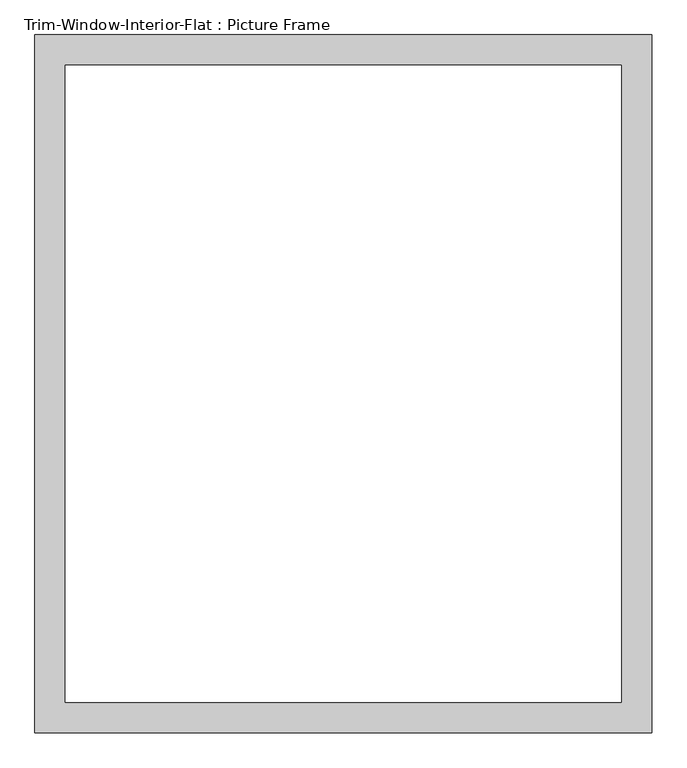
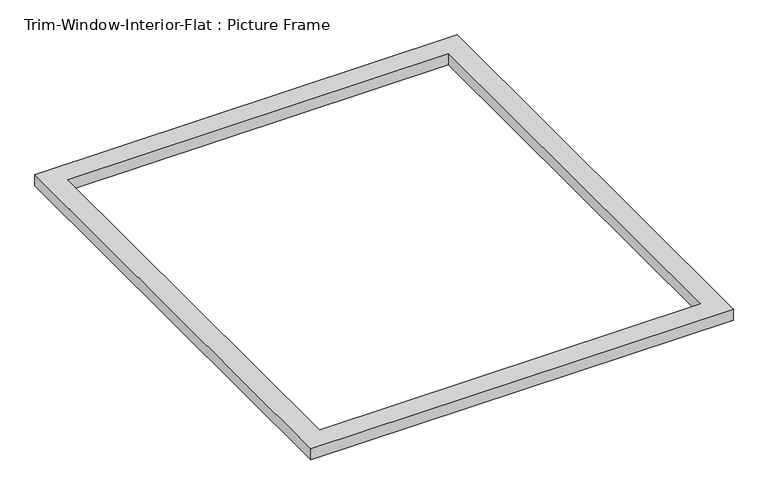
"""IFC4 building model written with IfcOpenShell, lengths in millimetres: proxy geometry, Trim-Window-Interior-Flat : Picture Frame."""

from ifc_helpers import new_model, si_unit, origin, origin_with_axes, place, context, project, spatial, polyline, outline, extrude, source, transform, mapped, element, save


def trim_window_interior_flat_picture_frame_2b4ba637(model_context):
    return source(origin(), model_context, "Body", "SweptSolid", [
        extrude(outline(polyline([(577.85, 44.45), (577.85, -1263.65), (-577.85, -1263.65), (-577.85, 44.45), (577.85, 44.45)]), holes=[polyline([(520.7, -12.7), (-520.7, -12.7), (-520.7, -1206.5), (520.7, -1206.5), (520.7, -12.7)])]), origin_with_axes(), (0.0, 0.0, 1.0), 31.75),
    ])


if __name__ == "__main__":
    model = new_model("IFC4")
    model_context = context("Model", 3, world=origin())
    ifc_project = project(units=[si_unit("LENGTHUNIT", "METRE", prefix="MILLI")], contexts=[model_context])
    site = spatial("IfcSite", under=ifc_project)
    building = spatial("IfcBuilding", under=site)
    placement = place(None, origin())
    trim_window_interior_flat_picture_frame_shape = trim_window_interior_flat_picture_frame_2b4ba637(model_context)
    element("IfcBuildingElementProxy", 1, Name="Trim-Window-Interior-Flat : Picture Frame", ObjectType="Trim-Window-Interior-Flat : Picture Frame", at=placement, inside=building, context=model_context, shape_type="MappedRepresentation", body=[
        mapped(trim_window_interior_flat_picture_frame_shape, transform((0.0, 0.0, 0.0), x_axis=(1.0, 0.0, 0.0), y_axis=(0.0, 1.0, 0.0), z_axis=(0.0, 0.0, 1.0))),
    ])
    save(model, "model.ifc")

# Revit data of these elements
# Type "Trim-Window-Interior-Flat : Picture Frame"
#   Trim Thickness_Picture Frame = 0' - 1 1/4"
#   Trim Width = 0' - 2 1/4"
#   Trim Thickness_with Sill = 0' - 0 3/4"
#   Sill Thickness = 0' - 1 1/4"
#   Opening Width [instance default] = 2' - 0"
#   Opening Height [instance default] = 3' - 0"
#   Default Elevation = 4' - 0"
#   Sill = no
#   Picture Frame = yes
#   Trim Material [instance default] = none
# Element 1 (IfcBuildingElementProxy, "Trim-Window-Interior-Flat : Picture Frame")
#   Opening Width = 3' - 6"
#   Opening Height = 4' - 0"
#   Trim Material = Wood - Stained
#   Materials on its faces: "Wood - Stained"
# Materials
#   "Wood - Stained": class "Wood", colour RGB 224 178 126, transparency 0, Cost = 0
